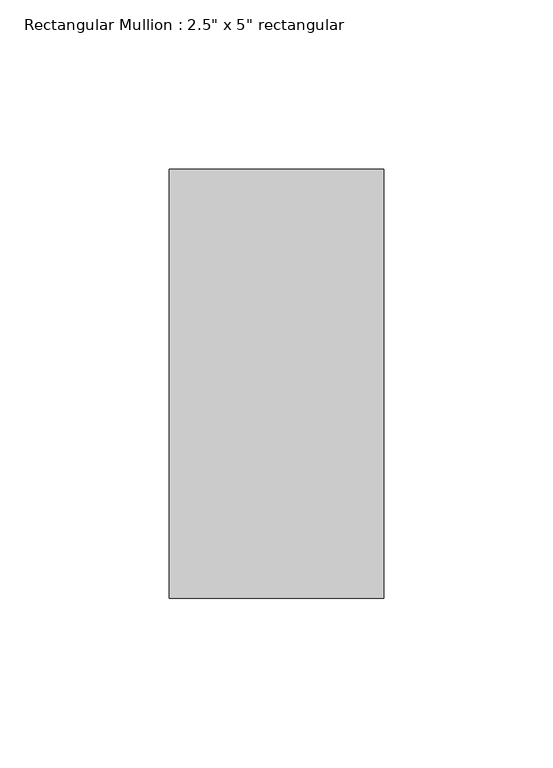
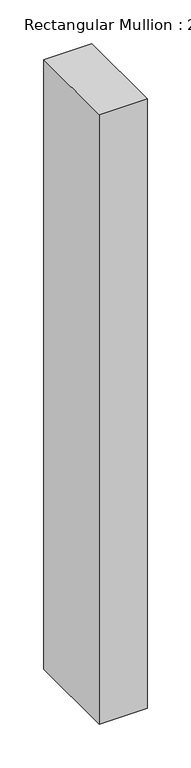
"""IFC4 building model written with IfcOpenShell, lengths in millimetres: member geometry."""

from ifc_helpers import new_model, si_unit, frame, origin, place, context, project, spatial, polyline, outline, extrude, source, transform, mapped, element, save


def member_ceefbd1b(model_context):
    return source(origin(), model_context, "Body", "SweptSolid", [
        extrude(outline(polyline([(0.0, 63.5), (0.0, -63.5), (-63.5, -63.5), (-63.5, 63.5), (0.0, 63.5)])), frame((0.0, 0.0, -851.3042254), z_axis=(0.0, 0.0, 1.0), x_axis=(1.0, 0.0, 0.0)), (0.0, 0.0, 1.0), 851.3042254),
    ])


if __name__ == "__main__":
    model = new_model("IFC4")
    model_context = context("Model", 3, world=origin())
    ifc_project = project(units=[si_unit("LENGTHUNIT", "METRE", prefix="MILLI")], contexts=[model_context])
    site = spatial("IfcSite", under=ifc_project)
    building = spatial("IfcBuilding", under=site)
    placement = place(None, origin())
    member_shape = member_ceefbd1b(model_context)
    element("IfcMember", 1, ObjectType="Rectangular Mullion : 2.5\" x 5\" rectangular", at=placement, inside=building, context=model_context, shape_type="MappedRepresentation", body=[
        mapped(member_shape, transform((0.0, 0.0, 0.0), x_axis=(1.0, 0.0, 0.0), y_axis=(0.0, 1.0, 0.0), z_axis=(0.0, 0.0, 1.0))),
    ])
    save(model, "model.ifc")

# Revit data of these elements
# Type "Rectangular Mullion : 2.5\" x 5\" rectangular"
#   built-in parameter 1007304 = 0.416667 (stored number, unit not read)
#   built-in parameter 1007301 = 0.104167 (stored number, unit not read)
#   built-in parameter 1007300 = 0.104167 (stored number, unit not read)
# Element 1 (IfcMember, "Rectangular Mullion : 2.5\" x 5\" rectangular")
#   Materials on its faces: "Aluminum"
# Materials
#   "Aluminum": class "Metal", colour RGB 247 247 247, transparency 0, Description = "Aluminum 6061", Cost = 0
